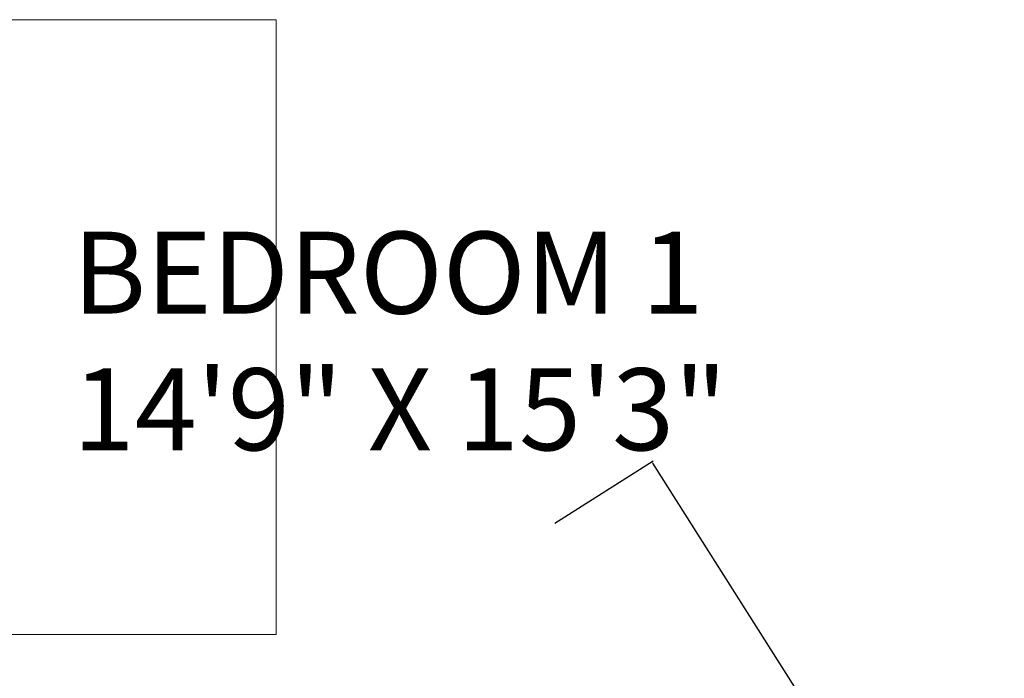
# Model space of a CAD drawing. Units: inches. Extents: x -4843 to -3402, y -164 to 3629.
# Tile 15 of 22: x -4532 to -4436, y 902 to 966. Entities that reach past the tile are written whole.
import ezdxf

# ---------------------------------------------------------------- set-up
doc = ezdxf.new("R2010")
doc.units = ezdxf.units.IN
for name, color, linetype, lineweight in [('A-ANNO-DIMS', 2, 'Continuous', 18), ('A-AREA-IDEN', 2, 'Continuous', 18), ('furniture', 6, 'Continuous', 18)]:
    doc.layers.add(name, color=color, linetype=linetype, lineweight=lineweight)
doc.styles.get("Standard").update_dxf_attribs({"font": 'arial.ttf'})
doc.dimstyles.get("Standard").update_dxf_attribs({"dimtxt": 0.18, "dimasz": 0.18, "dimexe": 0.18, "dimexo": 0.0625, "dimgap": 0.09, "dimtad": 0, "dimtih": 1, "dimtoh": 1, "dimdec": 4, "dimzin": 0, "dimdsep": 46, "dimtxsty": 'Standard', "dimcen": 0.09, "dimadec": 0, "dimazin": 0, "dimtfac": 1, "dimtdec": 4, "dimtofl": 0, "dimtmove": 0, "dimatfit": 3, "dimfxl": 1, "dimtolj": 1, "dimtzin": 0, "dimarcsym": 0})

# ---------------------------------------------------------------- blocks, each defined once
blk = doc.blocks.new('Bed - Queen')
for p, q in [((0, -80.00003), (0, 0)), ((0, 0), (59.99999, 0)), ((59.99999, 0), (59.99999, -80.00003)), ((7.99999, -1.2), (28.79998, -1.2)), ((7.99999, -14.4), (7.99999, -1.2)), ((28.79998, -1.2), (28.79998, -14.4)), ((31.19999, -1.2), (51.99999, -1.2)), ((31.19999, -14.4), (31.19999, -1.2)), ((51.99999, -1.2), (51.99999, -16.4)), ((0, -14.4), (44.8, -14.4)), ((59.99999, -29.6), (44.8, -14.4)), ((44.8, -14.4), (44.8, -29.6)), ((44.8, -16.8), (0, -16.8)), ((51.99999, -16.4), (46.79936, -16.4)), ((44.8, -29.6), (59.99999, -29.6)), ((59.99999, -80.00003), (0, -80.00003))]:
    blk.add_line(p, q)
blk = doc.blocks.new('*D51')
at = {"layer": 'A-ANNO-DIMS', "color": 0, "lineweight": -2, "transparency": 16777216}
for p, q in [((-4479.57, 916.866), (-4469.965, 922.969)), ((-4470.021, 922.721), (-4453.091, 896.074)), ((-4435.929, 869.063), (-4452.859, 895.71)), ((-4445.286, 862.905), (-4435.681, 869.008))]:
    blk.add_line(p, q, dxfattribs=at)
at = {"layer": 'A-ANNO-DIMS', "color": 0, "transparency": 16777216}
for points in [[(-4469.995, 922.737), (-4470.046, 922.704), (-4470.117, 922.872)], [(-4435.904, 869.079), (-4435.955, 869.047), (-4435.833, 868.911)]]:
    blk.add_solid(points, dxfattribs=at)
at = {"layer": 'Defpoints', "color": 0, "transparency": 16777216}
for p in [(-4479.623, 916.833), (-4435.833, 868.911), (-4445.339, 862.871)]:
    blk.add_point(p, dxfattribs=at)
at = {"layer": 'A-ANNO-DIMS', "color": 0, "transparency": 16777216, "insert": (-4452.975, 895.892), "char_height": 0.18, "attachment_point": 5}
blk.add_mtext('\\A1;64', dxfattribs=at)

msp = doc.modelspace()

# ---------------------------------------------------------------- block references
at = {"layer": 'furniture', "rotation": 90}
msp.add_blockref('Bed - Queen', (-4586.783, 906.016), dxfattribs=at)

# ---------------------------------------------------------------- texts
at = {"layer": 'A-AREA-IDEN', "insert": (-4526.64, 945.33), "char_height": 8, "attachment_point": 1}
msp.add_mtext_dynamic_manual_height_columns('BEDROOM 1\\P14\'9" X 15\'3"', width=66.87302, gutter_width=60, heights=[0], dxfattribs=at)

# ---------------------------------------------------------------- dimensions: what is measured, and where the dimension line sits
at = {"layer": 'A-ANNO-DIMS'}
dim = msp.add_linear_dim(base=(-4435.833, 868.911), p1=(-4479.623, 916.833), p2=(-4445.339, 862.871), angle=302.42984, dimstyle='Standard', override={"dimdec": 0, "dimlfac": 1, "dimrnd": 0, "dimzin": 0, "dimdsep": 46, "dimlunit": 2}, dxfattribs=at)
dim.commit()
dim.dimension.update_dxf_attribs({"geometry": '*D51', "text_midpoint": (-4452.975, 895.892)})

doc.saveas('drawing.dxf')
